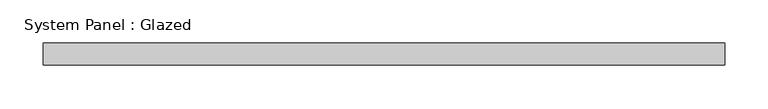
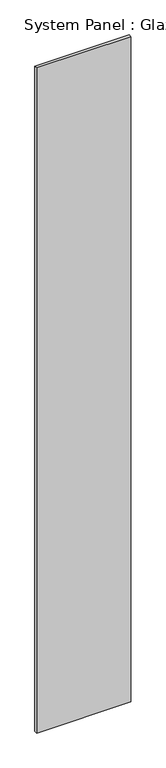
"""IFC4 building model written with IfcOpenShell, lengths in millimetres: plate geometry, System Panel : Glazed."""

from ifc_helpers import new_model, si_unit, origin, origin_with_axes, place, context, project, spatial, polyline, outline, extrude, source, transform, mapped, element, save


def system_panel_glazed_f7b0ce0e(model_context):
    return source(origin(), model_context, "Body", "SweptSolid", [
        extrude(outline(polyline([(393.7, 19.05), (-393.7, 19.05), (-393.7, 44.45), (393.7, 44.45), (393.7, 19.05)])), origin_with_axes(), (0.0, 0.0, 1.0), 5873.7551516),
    ])


if __name__ == "__main__":
    model = new_model("IFC4")
    model_context = context("Model", 3, world=origin())
    ifc_project = project(units=[si_unit("LENGTHUNIT", "METRE", prefix="MILLI")], contexts=[model_context])
    site = spatial("IfcSite", under=ifc_project)
    building = spatial("IfcBuilding", under=site)
    placement = place(None, origin())
    system_panel_glazed_shape = system_panel_glazed_f7b0ce0e(model_context)
    element("IfcPlate", 1, ObjectType="System Panel : Glazed", at=placement, inside=building, context=model_context, shape_type="MappedRepresentation", body=[
        mapped(system_panel_glazed_shape, transform((0.0, 0.0, 0.0), x_axis=(1.0, 0.0, 0.0), y_axis=(0.0, 1.0, 0.0), z_axis=(0.0, 0.0, 1.0))),
    ])
    save(model, "model.ifc")

# Revit data of these elements
# Type "System Panel : Glazed"
#   Construction Type Id = "GSP4R"
#   Analytic Construction = "1/8 in Pilkington single glazing"
#   Visual Light Transmittance = 0.9
#   Solar Heat Gain Coefficient = 0.86
#   Heat Transfer Coefficient (U) = 1.18115 BTU/(h·ft²·°F)
# Element 1 (IfcPlate, "System Panel : Glazed")
#   Materials on its faces: "Glass"
# Materials
#   "Glass": class "Glass", colour RGB 0 128 192, transparency 0.75, Description = "Soda Lime Glass", Cost = 0
